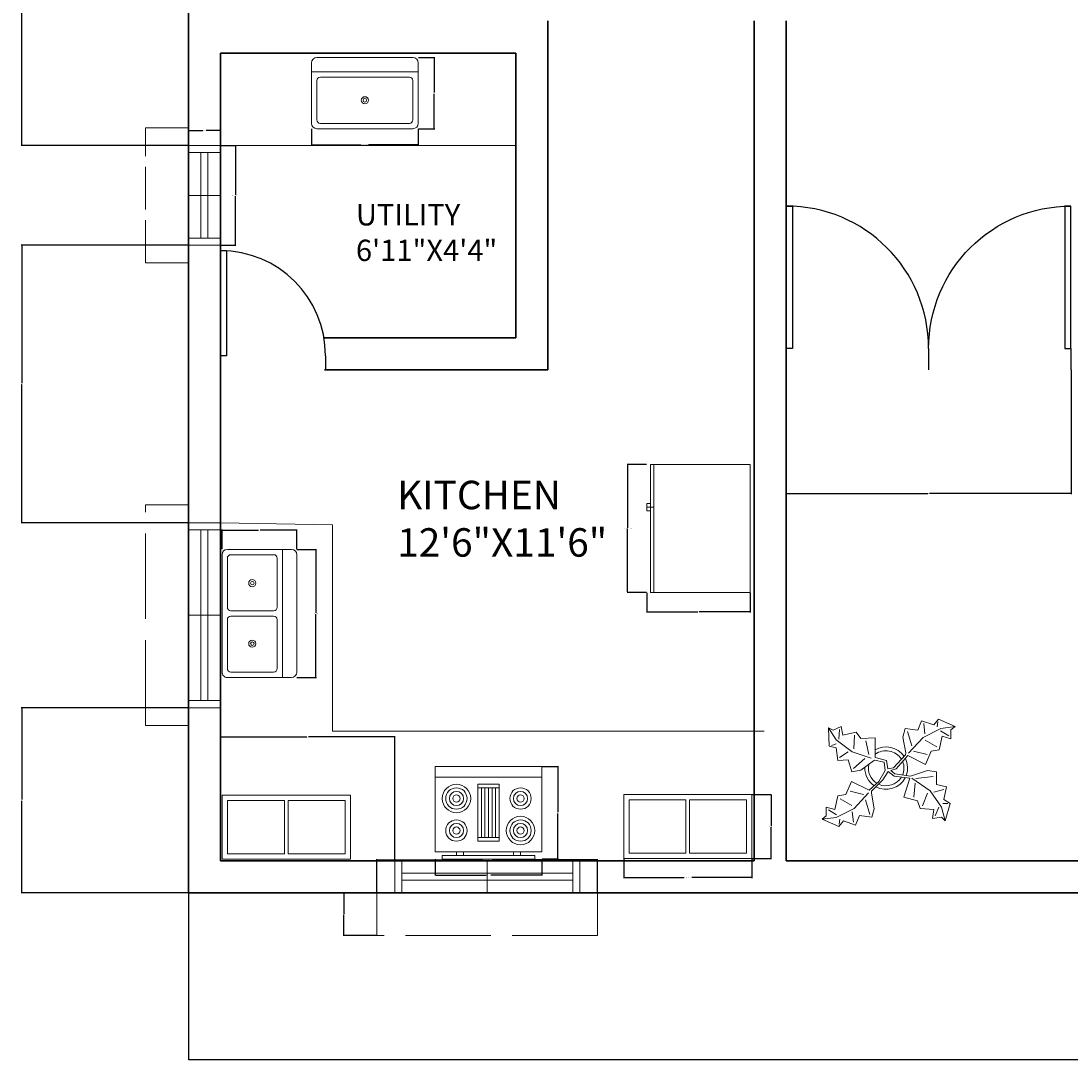
# Model space of a CAD drawing. Units: inches. Extents: x -1138 to 192, y 31 to 760.
# Tile 1 of 6: x -1138 to -843, y 31 to 323. Entities that reach past the tile are written whole.
import ezdxf

# ---------------------------------------------------------------- set-up
doc = ezdxf.new("R2010")
doc.units = ezdxf.units.IN
doc.header["$MEASUREMENT"] = 0
doc.linetypes.add('ACAD_ISO02W100', pattern=[15, 12, -3])
for name, color, linetype, lineweight in [('A-ANNO-DIMS', 2, 'Continuous', 18), ('A-AREA-IDEN', 7, 'Continuous', 18), ('A-DOOR', 3, 'Continuous', 25), ('A-EQPM', 8, 'Continuous', 18), ('A-FLOR-CASE', 32, 'Continuous', 18), ('A-FLOR-FIXT', 9, 'Continuous', 18), ('A-GLAZ', 4, 'Continuous', 20), ('A-GLAZ-OVHD', 4, 'ACAD_ISO02W100', 13), ('A-WALL', 7, 'Continuous', 35), ('L-PLNT', 94, 'Continuous', 18)]:
    doc.layers.add(name, color=color, linetype=linetype, lineweight=lineweight)
doc.styles.get("Standard").update_dxf_attribs({"font": 'arial.ttf'})
doc.dimstyles.get("Standard").update_dxf_attribs({"dimtxt": 0.18, "dimasz": 0.18, "dimexe": 0.18, "dimexo": 0.0625, "dimgap": 0.09, "dimtad": 0, "dimtih": 1, "dimtoh": 1, "dimdec": 1, "dimzin": 0, "dimdsep": 46, "dimlunit": 4, "dimtxsty": 'Standard', "dimcen": 0.09, "dimadec": 0, "dimazin": 0, "dimtfac": 1, "dimtdec": 1, "dimtofl": 0, "dimtmove": 0, "dimatfit": 3, "dimfxl": 1, "dimtolj": 1, "dimtzin": 0, "dimarcsym": 0})

# ---------------------------------------------------------------- blocks, each defined once
blk = doc.blocks.new('*U8')
for p, q in [((0, 0), (0, -100)), ((750, 0), (750, -100))]:
    blk.add_line(p, q)
blk.add_lwpolyline([(0, 0), (0, 750), (43.75, 750), (43.75, 0)], close=True)
blk.add_arc((0, 0), 750, 0, 90)
blk = doc.blocks.new('*U9')
for p, q in [((0, 0), (0, -6)), ((40, 0), (40, -6))]:
    blk.add_line(p, q)
blk.add_lwpolyline([(0, 0), (0, 40), (1.75, 40), (1.75, 0)], close=True)
blk.add_arc((0, 0), 40, 0, 90)
blk = doc.blocks.new('Plant - Rubber or Philodendron')
for p, q in [((-14.8639, 10.7964), (-12.6195, 11.8975)), ((-12.6195, 11.8975), (-12.1909, 9.4345)), ((8.8871, 10.7908), (9.9809, 13.4933)), ((9.9809, 13.4933), (13.3837, 12.301)), ((10.5828, 12.6946), (10.8893, 9.7953)), ((13.3837, 12.301), (14.68, 13.9039)), ((14.5816, 13.2037), (14.3848, 11.8033)), ((14.68, 13.9039), (19.3848, 11.8146)), ((19.3848, 11.8146), (15.3859, 11.3055)), ((19.3848, 11.8146), (18.1868, 10.9119)), ((-16.2005, 11.4774), (-13.9899, 8.1064)), ((-16.2005, 11.4774), (-14.8639, 10.7964)), ((-16.0159, 6.3329), (-16.2005, 11.4774)), ((-13.3174, 8.325), (-13.0735, 11.0065)), ((-12.1909, 9.4345), (-8.3829, 10.3)), ((-8.8369, 9.409), (-9.0894, 5.6095)), ((-8.3829, 10.3), (-7.0549, 8.501)), ((4.6914, 8.8812), (5.3859, 11.2828)), ((4.6914, 8.8812), (5.5014, 4.4831)), ((5.3859, 11.2828), (8.8871, 10.7908)), ((5.9878, 10.4842), (7.1971, 6.3869)), ((15.3859, 11.3055), (10.3916, 8.7942)), ((15.7909, 9.1065), (14.8995, 5.3044)), ((15.2875, 10.6053), (17.5907, 9.2105)), ((18.1925, 8.4119), (15.7909, 9.1065)), ((18.1868, 10.9119), (18.1925, 8.4119)), ((-14.0069, 5.8704), (-16.0159, 6.3329)), ((-15.3434, 6.5514), (-13.9984, 6.9884)), ((-13.9899, 8.1064), (-9.5434, 4.7185)), ((-7.0549, 8.501), (-3.0284, 8.6941)), ((-4.8529, 4.012), (-5.7184, 7.82)), ((-3.0284, 8.6941), (-3.0709, 3.1041)), ((10.3916, 8.7942), (6.2847, 4.4028)), ((14.2977, 6.1031), (10.9934, 7.9956)), ((-13.5868, 2.2894), (-14.0069, 5.8704)), ((-13.1329, 3.1804), (-10.6614, 4.727)), ((-9.5434, 4.7185), (-4.1917, 2.9888)), ((-3.0709, 3.1041), (0.0797, 2.3163)), ((2.1141, 0.2298), (5.4346, 3.9146)), ((6.1032, 3.6844), (2.8262, -0.031)), ((5.4346, 3.9146), (5.5014, 4.4831)), ((11.1089, 1.1958), (6.1032, 3.6844)), ((7.7005, 4.8881), (11.5025, 3.9967)), ((12.7005, 4.8994), (11.1089, 1.1958)), ((14.8995, 5.3044), (12.7005, 4.8994)), ((-10.6784, 2.491), (-13.5868, 2.2894)), ((-9.5858, -0.8715), (-10.6784, 2.491)), ((-9.1318, 0.0195), (-5.9793, 2.9025)), ((-7.1228, -0.443), (-3.5248, 2.2131)), ((-3.5248, 2.2131), (-3.3011, 2.4355)), ((-3.3011, 2.4355), (-0.5306, 1.7947)), ((-0.5306, 1.7947), (-0.2255, -0.5527)), ((-0.5306, 1.7947), (-0.5306, 1.7947)), ((0.0797, 2.3163), (0.4866, -0.031)), ((0.4866, -0.031), (2.1141, 0.2298)), ((-7.1228, -0.443), (-9.5858, -0.8715)), ((-2.019, -3.6148), (-0.2255, -0.5527)), ((-0.9375, -3.1608), (0.5883, -0.8135)), ((0.5883, -0.8135), (2.2447, -2.0916)), ((2.8262, -0.031), (1.3003, -0.5527)), ((1.3003, -0.5527), (2.4193, -1.4655)), ((2.2447, -2.0916), (6.7108, -2.6626)), ((2.4193, -1.4655), (6.895, -2.1175)), ((4.943, -7.9659), (6.7108, -2.6626)), ((11.6605, -0.5413), (6.895, -2.1175)), ((12.3677, -6.1981), (7.219, -2.6772)), ((8.3544, -2.7453), (13.1973, -2.1704)), ((11.6605, -0.5413), (14.1354, -0.8948)), ((14.1354, -0.8948), (14.1354, -4.4304)), ((-11.3237, -7.2629), (-9.7321, -3.5593)), ((-9.7321, -3.5593), (-4.7264, -6.0479)), ((-2.019, -3.6148), (-4.7264, -6.0479)), ((-4.0579, -6.2781), (-0.9375, -3.1608)), ((8.125, -4.0768), (7.7715, -7.9659)), ((16.2567, -5.8446), (13.4283, -6.5517)), ((14.1354, -4.4304), (16.9638, -5.1375)), ((16.9638, -5.1375), (16.2567, -8.673)), ((-14.4141, -11.4699), (-13.5228, -7.6679)), ((-13.5228, -7.6679), (-11.3237, -7.2629)), ((-12.921, -8.4665), (-9.6166, -10.359)), ((-6.3237, -7.2516), (-10.1257, -6.3602)), ((-9.0148, -11.1577), (-4.9047, -6.8122)), ((-4.611, -12.8477), (-5.8203, -8.7504)), ((-4.1246, -6.8466), (-4.0579, -6.2781)), ((-3.3146, -11.2447), (-4.1246, -6.8466)), ((8.8321, -9.0266), (4.943, -7.9659)), ((10.2463, -10.4408), (11.6605, -6.9053)), ((15.5496, -10.7943), (12.3677, -6.1981)), ((16.2567, -8.673), (18.0245, -9.7337)), ((-16.8157, -10.7754), (-14.4141, -11.4699)), ((-16.8101, -13.2754), (-16.8157, -10.7754)), ((-13.9107, -12.9688), (-16.2139, -11.574)), ((-14.0091, -13.669), (-9.0148, -11.1577)), ((-3.3146, -11.2447), (-4.0092, -13.6463)), ((9.5392, -11.1479), (8.8321, -9.0266)), ((13.4283, -11.5015), (9.5392, -11.1479)), ((13.0748, -13.9763), (13.4283, -11.5015)), ((14.8425, -10.7943), (13.7819, -13.2692)), ((16.6103, -14.6834), (15.5496, -10.7943)), ((17.3174, -9.7337), (15.9032, -9.7337)), ((18.0245, -9.7337), (16.6103, -14.6834)), ((-18.008, -14.1781), (-16.8101, -13.2754)), ((-18.008, -14.1781), (-14.0091, -13.669)), ((-13.3032, -16.2674), (-18.008, -14.1781)), ((-12.0069, -14.6645), (-13.3032, -16.2674)), ((-13.2048, -15.5672), (-13.008, -14.1668)), ((-8.6042, -15.8568), (-12.0069, -14.6645)), ((-9.206, -15.0581), (-9.5126, -12.1588)), ((-7.5103, -13.1543), (-8.6042, -15.8568)), ((-4.0092, -13.6463), (-7.5103, -13.1543)), ((15.5496, -13.6228), (13.0748, -13.9763)), ((16.6103, -14.6834), (15.5496, -13.6228))]:
    blk.add_line(p, q)
for centre, radius, start, end in [((0, 0), 6.1275, 34.37569, 120.1028), ((-0.0601, -0.2075), 5.2461, 33.82192, 124.9414), ((0.0308, 0.1664), 6, 178.6147, 235.1169), ((0.0308, 0.1664), 5, 168.1647, 238.6725), ((-0.2664, 0.1682), 5.2775, 338.4094, 20.03007), ((-0.098, 0.1364), 6.1288, 341.2017, 26.09184), ((-0.0234, 0.3825), 6.1492, 242.5812, 331.2714), ((-0.1102, 0.4886), 5.2883, 247.3711, 327.472)]:
    blk.add_arc(centre, radius, start, end)
blk = doc.blocks.new('Range-Oven - 30 in top')
for p, q in [((0, -3), (30, -3)), ((12, -6), (18, -6)), ((13, -20), (13, -6)), ((14, -6), (14, -20)), ((15, -20), (15, -6)), ((16, -6), (16, -20)), ((17, -20), (17, -6)), ((18, -20), (12, -20)), ((6, -24), (6, -25)), ((8, -25), (8, -24)), ((22, -25), (22, -24)), ((24, -24), (24, -25))]:
    blk.add_line(p, q)
for points in [[(0, -24), (0, 0), (30, 0), (30, -24)], [(12, -21), (12, -5), (18, -5), (18, -21)], [(2, -26), (2, -25), (28, -25), (28, -26)]]:
    blk.add_lwpolyline(points, close=True)
for centre, radius in [((6, -9), 4), ((6, -9), 3), ((6, -9), 2), ((6, -9), 1), ((24, -9), 3), ((24, -9), 2), ((24, -9), 1), ((24, -18), 4), ((6, -18), 3), ((6, -18), 2), ((6, -18), 1), ((24, -18), 3), ((24, -18), 2), ((24, -18), 1)]:
    blk.add_circle(centre, radius)
blk = doc.blocks.new('Refrigerator-2 door - 36 in top')
for p, q in [((0, -26.999999), (36, -26.999999)), ((11, -27.999999), (11, -28.999999)), ((11, -28.999999), (13, -28.999999)), ((12, -26.999999), (12, -28.999999)), ((13, -28.999999), (13, -27.999999))]:
    blk.add_line(p, q)
blk.add_lwpolyline([(0, -27.999999), (0, 0), (36, 0), (36, -27.999999)], close=True)
blk = doc.blocks.new('Sink-double - 36 in top')
for p, q in [((-18, -4), (18, -4)), ((-0.75, -18.5), (-0.75, -6.5)), ((0.75, -6.5), (0.75, -18.5))]:
    blk.add_line(p, q)
for points in [[(-16.5, 0), (16.5, 0)], [(-18, -19.5), (-18, -1.5)], [(18, -1.5), (18, -19.5)], [(-15.5, -5.5), (-1.75, -5.5)], [(1.75, -5.5), (15.5, -5.5)], [(-16.5, -18.5), (-16.5, -6.5)], [(16.5, -6.5), (16.5, -18.5)], [(-1.75, -19.5), (-15.5, -19.5)], [(15.5, -19.5), (1.75, -19.5)], [(16.5, -21), (-16.5, -21)]]:
    blk.add_lwpolyline(points)
for centre, radius in [((-8.5, -12.5), 1), ((8.5, -12.5), 1), ((-8.5, -12.5), 0.5), ((8.5, -12.5), 0.5)]:
    blk.add_circle(centre, radius)
for centre, radius, start, end in [((-16.5, -1.5), 1.5, 90, 180), ((16.5, -1.5), 1.5, 0, 90), ((-15.5, -6.5), 1, 90, 180), ((-1.75, -6.5), 1, 0, 90), ((1.75, -6.5), 1, 90, 180), ((15.5, -6.5), 1, 0, 90), ((-16.5, -19.5), 1.5, 180, 270), ((-15.5, -18.5), 1, 180, 270), ((-1.75, -18.5), 1, 270, 0), ((1.75, -18.5), 1, 180, 270), ((15.5, -18.5), 1, 270, 0), ((16.5, -19.5), 1.5, 270, 0)]:
    blk.add_arc(centre, radius, start, end)
blk = doc.blocks.new('Sink-single - 30 in top')
blk.add_line((-15, -3.999996), (15, -3.999996))
for points in [[(-13.5, 0), (13.5, 0)], [(-15, -18.499996), (-15, -1.5)], [(15, -1.5), (15, -18.499996)], [(-12.5, -5.499996), (12.5, -5.499996)], [(-13.5, -17.499996), (-13.5, -6.499996)], [(13.5, -6.499996), (13.5, -17.499996)], [(13.5, -19.999996), (-13.5, -19.999996)], [(12.5, -18.499996), (-12.5, -18.499996)]]:
    blk.add_lwpolyline(points)
for radius in [1, 0.5]:
    blk.add_circle((0, -11.999996), radius)
for centre, radius, start, end in [((-13.5, -1.5), 1.5, 90, 180), ((13.5, -1.5), 1.5, 0, 90), ((-12.5, -6.499996), 1, 90, 180), ((12.5, -6.499996), 1, 0, 90), ((-12.5, -17.499996), 1, 180, 270), ((12.5, -17.499996), 1, 270, 0), ((-13.5, -18.499996), 1.5, 180, 270), ((13.5, -18.499996), 1.5, 270, 0)]:
    blk.add_arc(centre, radius, start, end)
blk = doc.blocks.new('Wall Cabinet - 18 x 36 in front')
for p, q in [((17.5, -1.5), (17.5, -16.5)), ((18.5, -16.5), (18.5, -1.5))]:
    blk.add_line(p, q)
blk.add_lwpolyline([(0, -18), (0, 0), (36, 0), (36, -18)], close=True)
for points in [[(17.5, -16.5), (1.5, -16.5), (1.5, -1.5), (17.5, -1.5)], [(18.5, -1.5), (34.5, -1.5), (34.5, -16.5), (18.5, -16.5)]]:
    blk.add_lwpolyline(points)
blk = doc.blocks.new('WINDOW-48IN')
for p, q in [((0, 0), (0, 9)), ((2, 0), (2, 9)), ((26, 0), (26, 9)), ((50, 0), (50, 9)), ((52, 0), (52, 9)), ((2, 5.5), (50, 5.5)), ((2, 3.5), (50, 3.5))]:
    blk.add_line(p, q)
blk = doc.blocks.new('WINDOW-24IN')
for p, q in [((0, 0), (0, 9)), ((2, 0), (2, 9)), ((14, 0), (14, 9)), ((26, 0), (26, 9)), ((28, 0), (28, 9)), ((2, 5.5), (26, 5.5)), ((2, 3.5), (26, 3.5))]:
    blk.add_line(p, q)
blk = doc.blocks.new('WINDOW-PROJECTION-62IN')
at = {"ltscale": 2}
for p, q in [((0, 0), (0, 12)), ((0, 12), (62, 12)), ((62, 0), (62, 12)), ((5, 0), (0, 0)), ((57, 0), (62, 0))]:
    blk.add_line(p, q, dxfattribs=at)
blk = doc.blocks.new('WINDOW-PROJECTION-38IN')
for p, q in [((0, 0), (0, 12)), ((0, 12), (38, 12)), ((38, 0), (38, 12)), ((5, 0), (0, 0)), ((33, 0), (38, 0))]:
    blk.add_line(p, q)
blk = doc.blocks.new('*D47')
at = {"layer": 'A-ANNO-DIMS', "color": 0, "lineweight": -2, "transparency": 16777216}
for p, q in [((-1038.13, 77.88), (-1038.13, 87.29)), ((-1037.95, 87.11), (-1008.5, 87.11)), ((-976.31, 87.11), (-1005.76, 87.11)), ((-976.13, 77.88), (-976.13, 87.29))]:
    blk.add_line(p, q, dxfattribs=at)
at = {"layer": 'A-ANNO-DIMS', "color": 0, "transparency": 16777216}
for points in [[(-1037.95, 87.14), (-1037.95, 87.08), (-1038.13, 87.11)], [(-976.31, 87.14), (-976.31, 87.08), (-976.13, 87.11)]]:
    blk.add_solid(points, dxfattribs=at)
at = {"layer": 'Defpoints', "color": 0, "transparency": 16777216}
for p in [(-1038.13, 87.11), (-1038.13, 77.81), (-976.13, 77.81)]:
    blk.add_point(p, dxfattribs=at)
at = {"layer": 'A-ANNO-DIMS', "color": 0, "transparency": 16777216, "insert": (-1007.13, 87.11), "char_height": 0.18, "attachment_point": 5}
blk.add_mtext('\\A1;PROJECTION 62 TYP.', dxfattribs=at)
blk = doc.blocks.new('*D48')
at = {"layer": 'A-ANNO-DIMS', "color": 0, "lineweight": -2, "transparency": 16777216}
for p, q in [((-1038.2, 77.81), (-1047.61, 77.81)), ((-1047.43, 77.63), (-1047.43, 71.99)), ((-1047.43, 65.99), (-1047.43, 71.63)), ((-1038.2, 65.81), (-1047.61, 65.81))]:
    blk.add_line(p, q, dxfattribs=at)
at = {"layer": 'A-ANNO-DIMS', "color": 0, "transparency": 16777216}
for points in [[(-1047.46, 77.63), (-1047.4, 77.63), (-1047.43, 77.81)], [(-1047.46, 65.99), (-1047.4, 65.99), (-1047.43, 65.81)]]:
    blk.add_solid(points, dxfattribs=at)
at = {"layer": 'Defpoints', "color": 0, "transparency": 16777216}
for p in [(-1038.13, 77.81), (-1047.43, 65.81), (-1038.13, 65.81)]:
    blk.add_point(p, dxfattribs=at)
at = {"layer": 'A-ANNO-DIMS', "color": 0, "transparency": 16777216, "insert": (-1047.43, 71.81), "char_height": 0.18, "attachment_point": 5}
blk.add_mtext('\\A1;12 TYP.', dxfattribs=at)
blk = doc.blocks.new('*D49')
at = {"layer": 'A-ANNO-DIMS', "color": 0, "lineweight": -2, "transparency": 16777216}
for p, q in [((-1082.07, 287.81), (-1077.75, 287.81)), ((-1077.93, 287.63), (-1077.93, 274)), ((-1077.93, 259.99), (-1077.93, 273.63)), ((-1082.07, 259.81), (-1077.75, 259.81))]:
    blk.add_line(p, q, dxfattribs=at)
at = {"layer": 'A-ANNO-DIMS', "color": 0, "transparency": 16777216}
for points in [[(-1077.96, 287.63), (-1077.9, 287.63), (-1077.93, 287.81)], [(-1077.96, 259.99), (-1077.9, 259.99), (-1077.93, 259.81)]]:
    blk.add_solid(points, dxfattribs=at)
at = {"layer": 'Defpoints', "color": 0, "transparency": 16777216}
for p in [(-1082.13, 287.81), (-1082.13, 259.81), (-1077.93, 259.81)]:
    blk.add_point(p, dxfattribs=at)
at = {"layer": 'A-ANNO-DIMS', "color": 0, "transparency": 16777216, "insert": (-1077.93, 273.81), "char_height": 0.18, "attachment_point": 5}
blk.add_mtext('\\A1;WINDOW 28 TYP.', dxfattribs=at)
blk = doc.blocks.new('*D50')
at = {"layer": 'A-ANNO-DIMS', "color": 0, "lineweight": -2, "transparency": 16777216}
for p, q in [((-1091.13, 287.88), (-1091.13, 292.19)), ((-1082.13, 287.88), (-1082.13, 292.19)), ((-1090.95, 292.01), (-1087.09, 292.01)), ((-1082.31, 292.01), (-1086.17, 292.01))]:
    blk.add_line(p, q, dxfattribs=at)
at = {"layer": 'A-ANNO-DIMS', "color": 0, "transparency": 16777216}
for points in [[(-1090.95, 292.04), (-1090.95, 291.98), (-1091.13, 292.01)], [(-1082.31, 292.04), (-1082.31, 291.98), (-1082.13, 292.01)]]:
    blk.add_solid(points, dxfattribs=at)
at = {"layer": 'Defpoints', "color": 0, "transparency": 16777216}
for p in [(-1082.13, 292.01), (-1091.13, 287.81), (-1082.13, 287.81)]:
    blk.add_point(p, dxfattribs=at)
at = {"layer": 'A-ANNO-DIMS', "color": 0, "transparency": 16777216, "insert": (-1086.63, 292.01), "char_height": 0.18, "attachment_point": 5}
blk.add_mtext('\\A1;9 TYP.', dxfattribs=at)
blk = doc.blocks.new('*D61')
at = {"layer": 'A-ANNO-DIMS', "color": 0, "lineweight": -2, "transparency": 16777216}
for p, q in [((-968.82, 87.41), (-968.82, 81.89)), ((-932.82, 87.41), (-932.82, 81.89)), ((-968.64, 82.07), (-951.93, 82.07)), ((-933, 82.07), (-949.71, 82.07))]:
    blk.add_line(p, q, dxfattribs=at)
at = {"layer": 'A-ANNO-DIMS', "color": 0, "transparency": 16777216}
for points in [[(-968.64, 82.1), (-968.64, 82.04), (-968.82, 82.07)], [(-933, 82.1), (-933, 82.04), (-932.82, 82.07)]]:
    blk.add_solid(points, dxfattribs=at)
at = {"layer": 'Defpoints', "color": 0, "transparency": 16777216}
for p in [(-968.82, 87.47), (-932.82, 87.47), (-932.82, 82.07)]:
    blk.add_point(p, dxfattribs=at)
at = {"layer": 'A-ANNO-DIMS', "color": 0, "transparency": 16777216, "insert": (-950.82, 82.07), "char_height": 0.18, "attachment_point": 5}
blk.add_mtext('\\A1;CABINET 36 TYP.', dxfattribs=at)
blk = doc.blocks.new('*D62')
at = {"layer": 'A-ANNO-DIMS', "color": 0, "lineweight": -2, "transparency": 16777216}
for p, q in [((-932.76, 105.47), (-927.24, 105.47)), ((-927.42, 105.29), (-927.42, 96.65)), ((-927.42, 87.65), (-927.42, 96.29)), ((-932.76, 87.47), (-927.24, 87.47))]:
    blk.add_line(p, q, dxfattribs=at)
at = {"layer": 'A-ANNO-DIMS', "color": 0, "transparency": 16777216}
for points in [[(-927.45, 105.29), (-927.39, 105.29), (-927.42, 105.47)], [(-927.45, 87.65), (-927.39, 87.65), (-927.42, 87.47)]]:
    blk.add_solid(points, dxfattribs=at)
at = {"layer": 'Defpoints', "color": 0, "transparency": 16777216}
for p in [(-932.82, 105.47), (-927.42, 105.47), (-932.82, 87.47)]:
    blk.add_point(p, dxfattribs=at)
at = {"layer": 'A-ANNO-DIMS', "color": 0, "transparency": 16777216, "insert": (-927.42, 96.47), "char_height": 0.18, "attachment_point": 5}
blk.add_mtext('\\A1;18 TYP.', dxfattribs=at)
blk = doc.blocks.new('*D69')
at = {"layer": 'A-ANNO-DIMS', "color": 0, "lineweight": -2, "transparency": 16777216}
for p, q in [((-1021.8, 87.24), (-1021.8, 82.63)), ((-991.8, 87.24), (-991.8, 82.63)), ((-1021.62, 82.81), (-1007.5, 82.81)), ((-991.98, 82.81), (-1006.1, 82.81))]:
    blk.add_line(p, q, dxfattribs=at)
at = {"layer": 'A-ANNO-DIMS', "color": 0, "transparency": 16777216}
for points in [[(-1021.62, 82.84), (-1021.62, 82.78), (-1021.8, 82.81)], [(-991.98, 82.84), (-991.98, 82.78), (-991.8, 82.81)]]:
    blk.add_solid(points, dxfattribs=at)
at = {"layer": 'Defpoints', "color": 0, "transparency": 16777216}
for p in [(-1021.8, 87.31), (-991.8, 87.31), (-991.8, 82.81)]:
    blk.add_point(p, dxfattribs=at)
at = {"layer": 'A-ANNO-DIMS', "color": 0, "transparency": 16777216, "insert": (-1006.8, 82.81), "char_height": 0.18, "attachment_point": 5}
blk.add_mtext('\\A1;RANGE 30', dxfattribs=at)
blk = doc.blocks.new('*D70')
at = {"layer": 'A-ANNO-DIMS', "color": 0, "lineweight": -2, "transparency": 16777216}
for p, q in [((-991.74, 113.31), (-987.12, 113.31)), ((-987.3, 113.13), (-987.3, 100.49)), ((-987.3, 87.49), (-987.3, 100.12)), ((-991.74, 87.31), (-987.12, 87.31))]:
    blk.add_line(p, q, dxfattribs=at)
at = {"layer": 'A-ANNO-DIMS', "color": 0, "transparency": 16777216}
for points in [[(-987.33, 113.13), (-987.27, 113.13), (-987.3, 113.31)], [(-987.33, 87.49), (-987.27, 87.49), (-987.3, 87.31)]]:
    blk.add_solid(points, dxfattribs=at)
at = {"layer": 'Defpoints', "color": 0, "transparency": 16777216}
for p in [(-991.8, 113.31), (-987.3, 113.31), (-991.8, 87.31)]:
    blk.add_point(p, dxfattribs=at)
at = {"layer": 'A-ANNO-DIMS', "color": 0, "transparency": 16777216, "insert": (-987.3, 100.31), "char_height": 0.18, "attachment_point": 5}
blk.add_mtext('\\A1;26', dxfattribs=at)
blk = doc.blocks.new('*D71')
at = {"layer": 'A-ANNO-DIMS', "color": 0, "lineweight": -2, "transparency": 16777216}
for p, q in [((-962.36, 198.17), (-967.88, 198.17)), ((-967.7, 197.99), (-967.7, 180.36)), ((-967.7, 162.35), (-967.7, 179.99)), ((-962.36, 162.17), (-967.88, 162.17))]:
    blk.add_line(p, q, dxfattribs=at)
at = {"layer": 'A-ANNO-DIMS', "color": 0, "transparency": 16777216}
for points in [[(-967.73, 197.99), (-967.67, 197.99), (-967.7, 198.17)], [(-967.73, 162.35), (-967.67, 162.35), (-967.7, 162.17)]]:
    blk.add_solid(points, dxfattribs=at)
at = {"layer": 'Defpoints', "color": 0, "transparency": 16777216}
for p in [(-962.3, 198.17), (-967.7, 162.17), (-962.3, 162.17)]:
    blk.add_point(p, dxfattribs=at)
at = {"layer": 'A-ANNO-DIMS', "color": 0, "transparency": 16777216, "insert": (-967.7, 180.17), "char_height": 0.18, "attachment_point": 5}
blk.add_mtext('\\A1;REFRIGERATOR 36', dxfattribs=at)
blk = doc.blocks.new('*D72')
at = {"layer": 'A-ANNO-DIMS', "color": 0, "lineweight": -2, "transparency": 16777216}
for p, q in [((-962.3, 162.11), (-962.3, 156.59)), ((-933.3, 162.11), (-933.3, 156.59)), ((-962.12, 156.77), (-948.02, 156.77)), ((-933.48, 156.77), (-947.58, 156.77))]:
    blk.add_line(p, q, dxfattribs=at)
at = {"layer": 'A-ANNO-DIMS', "color": 0, "transparency": 16777216}
for points in [[(-962.12, 156.8), (-962.12, 156.74), (-962.3, 156.77)], [(-933.48, 156.8), (-933.48, 156.74), (-933.3, 156.77)]]:
    blk.add_solid(points, dxfattribs=at)
at = {"layer": 'Defpoints', "color": 0, "transparency": 16777216}
for p in [(-962.3, 162.17), (-933.3, 162.17), (-933.3, 156.77)]:
    blk.add_point(p, dxfattribs=at)
at = {"layer": 'A-ANNO-DIMS', "color": 0, "transparency": 16777216, "insert": (-947.8, 156.77), "char_height": 0.18, "attachment_point": 5}
blk.add_mtext('\\A1;29', dxfattribs=at)
blk = doc.blocks.new('*D73')
at = {"layer": 'A-ANNO-DIMS', "color": 0, "lineweight": -2, "transparency": 16777216}
for p, q in [((-1060.61, 174.32), (-1055.09, 174.32)), ((-1055.27, 174.14), (-1055.27, 156.51)), ((-1055.27, 138.5), (-1055.27, 156.14)), ((-1060.61, 138.32), (-1055.09, 138.32))]:
    blk.add_line(p, q, dxfattribs=at)
at = {"layer": 'A-ANNO-DIMS', "color": 0, "transparency": 16777216}
for points in [[(-1055.3, 174.14), (-1055.24, 174.14), (-1055.27, 174.32)], [(-1055.3, 138.5), (-1055.24, 138.5), (-1055.27, 138.32)]]:
    blk.add_solid(points, dxfattribs=at)
at = {"layer": 'Defpoints', "color": 0, "transparency": 16777216}
for p in [(-1060.67, 174.32), (-1060.67, 138.32), (-1055.27, 138.32)]:
    blk.add_point(p, dxfattribs=at)
at = {"layer": 'A-ANNO-DIMS', "color": 0, "transparency": 16777216, "insert": (-1055.27, 156.32), "char_height": 0.18, "attachment_point": 5}
blk.add_mtext('\\A1;SINK 36', dxfattribs=at)
blk = doc.blocks.new('*D74')
at = {"layer": 'A-ANNO-DIMS', "color": 0, "lineweight": -2, "transparency": 16777216}
for p, q in [((-1081.67, 174.39), (-1081.67, 179.9)), ((-1081.49, 179.72), (-1071.38, 179.72)), ((-1060.85, 179.72), (-1070.97, 179.72)), ((-1060.67, 174.39), (-1060.67, 179.9))]:
    blk.add_line(p, q, dxfattribs=at)
at = {"layer": 'A-ANNO-DIMS', "color": 0, "transparency": 16777216}
for points in [[(-1081.49, 179.75), (-1081.49, 179.69), (-1081.67, 179.72)], [(-1060.85, 179.75), (-1060.85, 179.69), (-1060.67, 179.72)]]:
    blk.add_solid(points, dxfattribs=at)
at = {"layer": 'Defpoints', "color": 0, "transparency": 16777216}
for p in [(-1060.67, 179.72), (-1081.67, 174.32), (-1060.67, 174.32)]:
    blk.add_point(p, dxfattribs=at)
at = {"layer": 'A-ANNO-DIMS', "color": 0, "transparency": 16777216, "insert": (-1071.17, 179.72), "char_height": 0.18, "attachment_point": 5}
blk.add_mtext('\\A1;21', dxfattribs=at)
blk = doc.blocks.new('*D75')
at = {"layer": 'A-ANNO-DIMS', "color": 0, "lineweight": -2, "transparency": 16777216}
for p, q in [((-1056.54, 292.48), (-1056.54, 287.87)), ((-1026.54, 292.48), (-1026.54, 287.87)), ((-1056.36, 288.05), (-1042.58, 288.05)), ((-1026.72, 288.05), (-1040.49, 288.05))]:
    blk.add_line(p, q, dxfattribs=at)
at = {"layer": 'A-ANNO-DIMS', "color": 0, "transparency": 16777216}
for points in [[(-1056.36, 288.08), (-1056.36, 288.02), (-1056.54, 288.05)], [(-1026.72, 288.08), (-1026.72, 288.02), (-1026.54, 288.05)]]:
    blk.add_solid(points, dxfattribs=at)
at = {"layer": 'Defpoints', "color": 0, "transparency": 16777216}
for p in [(-1056.54, 292.55), (-1026.54, 292.55), (-1026.54, 288.05)]:
    blk.add_point(p, dxfattribs=at)
at = {"layer": 'A-ANNO-DIMS', "color": 0, "transparency": 16777216, "insert": (-1041.54, 288.05), "char_height": 0.18, "attachment_point": 5}
blk.add_mtext('\\A1;UTILITY SINK 30', dxfattribs=at)
blk = doc.blocks.new('*D76')
at = {"layer": 'A-ANNO-DIMS', "color": 0, "lineweight": -2, "transparency": 16777216}
for p, q in [((-1026.47, 312.55), (-1021.86, 312.55)), ((-1022.04, 312.37), (-1022.04, 302.73)), ((-1022.04, 292.73), (-1022.04, 302.36)), ((-1026.47, 292.55), (-1021.86, 292.55))]:
    blk.add_line(p, q, dxfattribs=at)
at = {"layer": 'A-ANNO-DIMS', "color": 0, "transparency": 16777216}
for points in [[(-1022.07, 312.37), (-1022.01, 312.37), (-1022.04, 312.55)], [(-1022.07, 292.73), (-1022.01, 292.73), (-1022.04, 292.55)]]:
    blk.add_solid(points, dxfattribs=at)
at = {"layer": 'Defpoints', "color": 0, "transparency": 16777216}
for p in [(-1026.54, 312.55), (-1022.04, 312.55), (-1026.54, 292.55)]:
    blk.add_point(p, dxfattribs=at)
at = {"layer": 'A-ANNO-DIMS', "color": 0, "transparency": 16777216, "insert": (-1022.04, 302.55), "char_height": 0.18, "attachment_point": 5}
blk.add_mtext('\\A1;20', dxfattribs=at)
blk = doc.blocks.new('*D85')
at = {"layer": 'A-ANNO-DIMS', "color": 0, "lineweight": -2, "transparency": 16777216}
for p, q in [((-1091.13, 77.75), (-1091.13, 30.82)), ((-514.13, 77.75), (-514.13, 30.82)), ((-1090.95, 31), (-802.92, 31)), ((-514.31, 31), (-802.34, 31))]:
    blk.add_line(p, q, dxfattribs=at)
at = {"layer": 'A-ANNO-DIMS', "color": 0, "transparency": 16777216}
for points in [[(-1090.95, 31.03), (-1090.95, 30.97), (-1091.13, 31)], [(-514.31, 31.03), (-514.31, 30.97), (-514.13, 31)]]:
    blk.add_solid(points, dxfattribs=at)
at = {"layer": 'Defpoints', "color": 0, "transparency": 16777216}
for p in [(-1091.13, 77.81), (-514.13, 77.81), (-514.13, 31)]:
    blk.add_point(p, dxfattribs=at)
at = {"layer": 'A-ANNO-DIMS', "color": 0, "transparency": 16777216, "insert": (-802.63, 31), "char_height": 0.18, "attachment_point": 5}
blk.add_mtext('\\A1;577', dxfattribs=at)
blk = doc.blocks.new('*D92')
at = {"layer": 'A-ANNO-DIMS', "color": 0, "lineweight": -2, "transparency": 16777216}
for p, q in [((-1091.2, 129.81), (-1138.13, 129.81)), ((-1137.95, 129.63), (-1137.95, 103.99)), ((-1137.95, 77.99), (-1137.95, 103.63)), ((-1091.2, 77.81), (-1138.13, 77.81))]:
    blk.add_line(p, q, dxfattribs=at)
at = {"layer": 'A-ANNO-DIMS', "color": 0, "transparency": 16777216}
for points in [[(-1137.98, 129.63), (-1137.92, 129.63), (-1137.95, 129.81)], [(-1137.98, 77.99), (-1137.92, 77.99), (-1137.95, 77.81)]]:
    blk.add_solid(points, dxfattribs=at)
at = {"layer": 'Defpoints', "color": 0, "transparency": 16777216}
for p in [(-1137.95, 129.81), (-1091.13, 129.81), (-1091.13, 77.81)]:
    blk.add_point(p, dxfattribs=at)
at = {"layer": 'A-ANNO-DIMS', "color": 0, "transparency": 16777216, "insert": (-1137.95, 103.81), "char_height": 0.18, "attachment_point": 5}
blk.add_mtext('\\A1;52', dxfattribs=at)
blk = doc.blocks.new('*D93')
at = {"layer": 'A-ANNO-DIMS', "color": 0, "lineweight": -2, "transparency": 16777216}
for p, q in [((-1091.2, 259.81), (-1138.13, 259.81)), ((-1137.95, 259.63), (-1137.95, 220.99)), ((-1137.95, 181.99), (-1137.95, 220.63)), ((-1091.2, 181.81), (-1138.13, 181.81))]:
    blk.add_line(p, q, dxfattribs=at)
at = {"layer": 'A-ANNO-DIMS', "color": 0, "transparency": 16777216}
for points in [[(-1137.98, 259.63), (-1137.92, 259.63), (-1137.95, 259.81)], [(-1137.98, 181.99), (-1137.92, 181.99), (-1137.95, 181.81)]]:
    blk.add_solid(points, dxfattribs=at)
at = {"layer": 'Defpoints', "color": 0, "transparency": 16777216}
for p in [(-1137.95, 259.81), (-1091.13, 259.81), (-1091.13, 181.81)]:
    blk.add_point(p, dxfattribs=at)
at = {"layer": 'A-ANNO-DIMS', "color": 0, "transparency": 16777216, "insert": (-1137.95, 220.81), "char_height": 0.18, "attachment_point": 5}
blk.add_mtext('\\A1;78', dxfattribs=at)
blk = doc.blocks.new('*D94')
at = {"layer": 'A-ANNO-DIMS', "color": 0, "lineweight": -2, "transparency": 16777216}
for p, q in [((-1091.2, 565.81), (-1138.13, 565.81)), ((-1137.95, 565.63), (-1137.95, 426.99)), ((-1137.95, 287.99), (-1137.95, 426.63)), ((-1091.2, 287.81), (-1138.13, 287.81))]:
    blk.add_line(p, q, dxfattribs=at)
at = {"layer": 'A-ANNO-DIMS', "color": 0, "transparency": 16777216}
for points in [[(-1137.98, 565.63), (-1137.92, 565.63), (-1137.95, 565.81)], [(-1137.98, 287.99), (-1137.92, 287.99), (-1137.95, 287.81)]]:
    blk.add_solid(points, dxfattribs=at)
at = {"layer": 'Defpoints', "color": 0, "transparency": 16777216}
for p in [(-1137.95, 565.81), (-1091.13, 565.81), (-1091.13, 287.81)]:
    blk.add_point(p, dxfattribs=at)
at = {"layer": 'A-ANNO-DIMS', "color": 0, "transparency": 16777216, "insert": (-1137.95, 426.81), "char_height": 0.18, "attachment_point": 5}
blk.add_mtext('\\A1;278', dxfattribs=at)
blk = doc.blocks.new('*D97')
at = {"layer": 'A-ANNO-DIMS', "color": 0, "lineweight": -2, "transparency": 16777216}
for p, q in [((-1082.13, 86.88), (-1082.13, 121.81)), ((-1081.95, 121.63), (-1057.86, 121.63)), ((-1033.31, 121.63), (-1057.41, 121.63)), ((-1033.13, 86.88), (-1033.13, 121.81))]:
    blk.add_line(p, q, dxfattribs=at)
at = {"layer": 'A-ANNO-DIMS', "color": 0, "transparency": 16777216}
for points in [[(-1081.95, 121.66), (-1081.95, 121.6), (-1082.13, 121.63)], [(-1033.31, 121.66), (-1033.31, 121.6), (-1033.13, 121.63)]]:
    blk.add_solid(points, dxfattribs=at)
at = {"layer": 'Defpoints', "color": 0, "transparency": 16777216}
for p in [(-1033.13, 121.63), (-1082.13, 86.81), (-1033.13, 86.81)]:
    blk.add_point(p, dxfattribs=at)
at = {"layer": 'A-ANNO-DIMS', "color": 0, "transparency": 16777216, "insert": (-1057.63, 121.63), "char_height": 0.18, "attachment_point": 5}
blk.add_mtext('\\A1;49', dxfattribs=at)
blk = doc.blocks.new('*D98')
at = {"layer": 'A-ANNO-DIMS', "color": 0, "lineweight": -2, "transparency": 16777216}
for p, q in [((-923.13, 224.75), (-923.13, 189.82)), ((-843.13, 224.75), (-843.13, 189.82)), ((-922.95, 190), (-883.35, 190)), ((-843.31, 190), (-882.91, 190))]:
    blk.add_line(p, q, dxfattribs=at)
at = {"layer": 'A-ANNO-DIMS', "color": 0, "transparency": 16777216}
for points in [[(-922.95, 190.03), (-922.95, 189.97), (-923.13, 190)], [(-843.31, 190.03), (-843.31, 189.97), (-843.13, 190)]]:
    blk.add_solid(points, dxfattribs=at)
at = {"layer": 'Defpoints', "color": 0, "transparency": 16777216}
for p in [(-923.13, 224.81), (-843.13, 224.81), (-923.13, 190)]:
    blk.add_point(p, dxfattribs=at)
at = {"layer": 'A-ANNO-DIMS', "color": 0, "transparency": 16777216, "insert": (-883.13, 190), "char_height": 0.18, "attachment_point": 5}
blk.add_mtext('\\A1;80', dxfattribs=at)

msp = doc.modelspace()

# ---------------------------------------------------------------- linework, layer by layer
at = {"layer": 'A-FLOR-CASE'}
for p, q in [((-1082.133, 287.813), (-999.133, 287.813)), ((-1050.618, 181.262), (-1082.133, 181.813)), ((-1050.618, 123.222), (-1050.618, 181.262)), ((-929.385, 123.222), (-1050.618, 123.222))]:
    msp.add_line(p, q, dxfattribs=at)
at = {"layer": 'A-WALL'}
for p, q in [((-1091.133, 491.813), (-1091.133, 294.813)), ((-990.133, 224.813), (-990.133, 322.813)), ((-932.133, 86.813), (-932.133, 322.813)), ((-923.133, 313.813), (-923.133, 322.813)), ((-1091.133, 313.813), (-1091.133, 233.813)), ((-1082.133, 313.813), (-1082.133, 224.813)), ((-999.133, 313.813), (-1082.133, 313.813)), ((-1082.133, 313.813), (-1082.133, 294.813)), ((-999.133, 233.813), (-999.133, 313.813)), ((-923.133, 233.813), (-923.133, 313.813)), ((-1091.133, 233.813), (-1091.133, 77.813)), ((-1053.043, 233.813), (-999.133, 233.813)), ((-1053.043, 233.813), (-999.133, 233.813)), ((-923.133, 224.813), (-923.133, 233.813)), ((-883.245, 233.813), (-883.02, 233.813)), ((-1082.133, 224.813), (-1082.133, 86.813)), ((-1052.869, 224.813), (-990.133, 224.813)), ((-923.133, 86.813), (-923.133, 224.813)), ((-1082.133, 86.813), (-932.133, 86.813)), ((-923.133, 86.813), (-523.133, 86.813)), ((-1091.133, 77.813), (-514.133, 77.813))]:
    msp.add_line(p, q, dxfattribs=at)

# ---------------------------------------------------------------- block references
at = {"layer": 'A-DOOR'}
msp.add_blockref('*U9', (-923.133, 230.813), dxfattribs=at)
at = {"layer": 'A-DOOR', "xscale": -1}
msp.add_blockref('*U9', (-843.133, 230.813), dxfattribs=at)
at = {"layer": 'A-DOOR', "xscale": 0.0393700787401575, "yscale": 0.0393700787401575, "zscale": 0.0393700787401575}
msp.add_blockref('*U8', (-1082.133, 228.75), dxfattribs=at)
at = {"layer": 'A-EQPM', "rotation": 270}
msp.add_blockref('Refrigerator-2 door - 36 in top', (-933.298, 198.173), dxfattribs=at)
at = {"layer": 'A-EQPM'}
msp.add_blockref('Range-Oven - 30 in top', (-1021.801, 113.306), dxfattribs=at)
at = {"layer": 'A-FLOR-CASE'}
for p in [(-1081.586, 105.25), (-968.819, 105.472)]:
    msp.add_blockref('Wall Cabinet - 18 x 36 in front', p, dxfattribs=at)
at = {"layer": 'A-FLOR-FIXT'}
msp.add_blockref('Sink-single - 30 in top', (-1041.536, 312.545), dxfattribs=at)
at = {"layer": 'A-FLOR-FIXT', "rotation": 270}
msp.add_blockref('Sink-double - 36 in top', (-1060.673, 156.324), dxfattribs=at)
at = {"layer": 'A-GLAZ'}
for name, p, rotation in [('WINDOW-24IN', (-1091.133, 287.813), 270.0000000000017), ('WINDOW-48IN', (-1091.133, 181.813), 270.0000000000009)]:
    msp.add_blockref(name, p, dxfattribs=dict(at, rotation=rotation))
msp.add_blockref('WINDOW-48IN', (-1033.133, 77.813), dxfattribs=at)
at = {"layer": 'A-GLAZ-OVHD'}
for name, p, rotation in [('WINDOW-PROJECTION-38IN', (-1091.133, 254.813), 89.99999999999905), ('WINDOW-PROJECTION-62IN', (-1091.133, 124.813), 89.9999999999993), ('WINDOW-PROJECTION-62IN', (-976.133, 77.813), 180)]:
    msp.add_blockref(name, p, dxfattribs=dict(at, rotation=rotation))
at = {"layer": 'L-PLNT'}
msp.add_blockref('Plant - Rubber or Philodendron', (-895.084, 112.684), dxfattribs=at)

# ---------------------------------------------------------------- texts
at = {"layer": 'A-AREA-IDEN', "attachment_point": 1}
for s, insert, char_height in [('UTILITY\\P6\'11"X4\'4"', (-1044.049, 271.358), 6), ('KITCHEN\\P12\'6"X11\'6"', (-1032.465, 193.604), 8)]:
    msp.add_mtext_dynamic_manual_height_columns(s, width=126.58932, gutter_width=1, heights=[0], dxfattribs=dict(at, insert=insert, char_height=char_height))

# ---------------------------------------------------------------- dimensions: what is measured, and where the dimension line sits
at = {"layer": 'A-ANNO-DIMS'}
for base, p1, p2, angle, picture, middle in [((-1137.948, 565.813), (-1091.133, 287.813), (-1091.133, 565.813), 90, '*D94', (-1137.948, 426.813)), ((-1022.036, 312.545), (-1026.536, 292.545), (-1026.536, 312.545), 90, '*D76', (-1022.036, 302.545)), ((-1137.948, 259.813), (-1091.133, 181.813), (-1091.133, 259.813), 90, '*D93', (-1137.948, 220.813)), ((-923.133, 189.998), (-843.133, 224.813), (-923.133, 224.813), 180, '*D98', (-883.133, 189.998)), ((-1137.948, 129.813), (-1091.133, 77.813), (-1091.133, 129.813), 90, '*D92', (-1137.948, 103.813)), ((-1033.133, 121.628), (-1082.133, 86.813), (-1033.133, 86.813), 0, '*D97', (-1057.633, 121.628)), ((-987.301, 113.306), (-991.801, 87.306), (-991.801, 113.306), 90, '*D70', (-987.301, 100.306))]:
    dim = msp.add_linear_dim(base=base, p1=p1, p2=p2, angle=angle, dimstyle='Standard', override={"dimdec": 0, "dimlfac": 1, "dimrnd": 0, "dimzin": 0, "dimdsep": 46, "dimlunit": 2}, dxfattribs=at)
    dim.commit()
    dim.dimension.update_dxf_attribs({"geometry": picture, "text_midpoint": middle})
for base, p1, p2, angle, text, picture, middle in [((-1082.133, 292.013), (-1091.133, 287.813), (-1082.133, 287.813), 0, '<> TYP.', '*D50', (-1086.633, 292.013)), ((-1077.933, 259.813), (-1082.133, 287.813), (-1082.133, 259.813), 270, 'WINDOW <> TYP.', '*D49', (-1077.933, 273.813)), ((-967.698, 162.173), (-962.298, 198.173), (-962.298, 162.173), 270, 'REFRIGERATOR <>', '*D71', (-967.698, 180.173)), ((-1055.273, 138.324), (-1060.673, 174.324), (-1060.673, 138.324), 270, 'SINK <>', '*D73', (-1055.273, 156.324)), ((-927.419, 105.472), (-932.819, 87.472), (-932.819, 105.472), 90, '<> TYP.', '*D62', (-927.419, 96.472)), ((-1038.133, 87.113), (-976.133, 77.813), (-1038.133, 77.813), 180, 'PROJECTION <> TYP.', '*D47', (-1007.133, 87.113)), ((-1047.433, 65.813), (-1038.133, 77.813), (-1038.133, 65.813), 270, '<> TYP.', '*D48', (-1047.433, 71.813))]:
    dim = msp.add_linear_dim(base=base, p1=p1, p2=p2, angle=angle, text=text, dimstyle='Standard', override={"dimdec": 0, "dimlfac": 1, "dimrnd": 0, "dimzin": 0, "dimdsep": 46, "dimlunit": 2}, dxfattribs=at)
    dim.commit()
    dim.dimension.update_dxf_attribs({"geometry": picture, "text_midpoint": middle})
for base, p1, p2, text, picture, middle in [((-1026.536, 288.045), (-1056.536, 292.545), (-1026.536, 292.545), 'UTILITY SINK <>', '*D75', (-1041.536, 288.045)), ((-991.801, 82.806), (-1021.801, 87.306), (-991.801, 87.306), 'RANGE <>', '*D69', (-1006.801, 82.806)), ((-932.819, 82.072), (-968.819, 87.472), (-932.819, 87.472), 'CABINET <> TYP.', '*D61', (-950.819, 82.072))]:
    dim = msp.add_linear_dim(base=base, p1=p1, p2=p2, text=text, dimstyle='Standard', override={"dimdec": 0, "dimlfac": 1, "dimrnd": 0, "dimzin": 0, "dimdsep": 46, "dimlunit": 2}, dxfattribs=at)
    dim.commit()
    dim.dimension.update_dxf_attribs({"geometry": picture, "text_midpoint": middle})
for base, p1, p2, picture, middle in [((-1060.673, 179.724), (-1081.673, 174.324), (-1060.673, 174.324), '*D74', (-1071.173, 179.724)), ((-933.298, 156.773), (-962.298, 162.173), (-933.298, 162.173), '*D72', (-947.798, 156.773)), ((-514.133, 30.998), (-1091.133, 77.813), (-514.133, 77.813), '*D85', (-802.633, 30.998))]:
    dim = msp.add_linear_dim(base=base, p1=p1, p2=p2, dimstyle='Standard', override={"dimdec": 0, "dimlfac": 1, "dimrnd": 0, "dimzin": 0, "dimdsep": 46, "dimlunit": 2}, dxfattribs=at)
    dim.commit()
    dim.dimension.update_dxf_attribs({"geometry": picture, "text_midpoint": middle})

doc.saveas('drawing.dxf')
